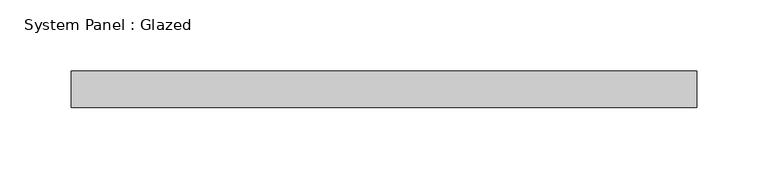
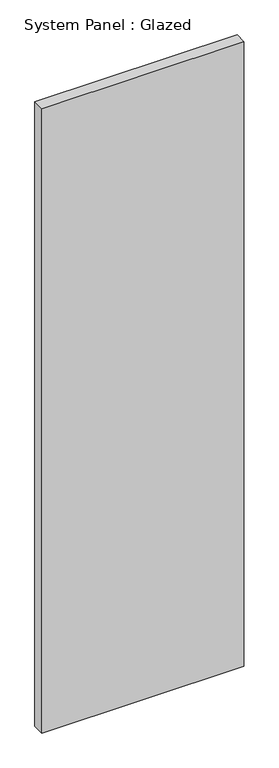
"""IFC4 building model written with IfcOpenShell, lengths in millimetres: plate geometry, System Panel : Glazed."""

from ifc_helpers import new_model, si_unit, origin, origin_with_axes, place, context, project, spatial, polyline, outline, extrude, source, transform, mapped, element, save


def system_panel_glazed_5472c3c5(model_context):
    return source(origin(), model_context, "Body", "SweptSolid", [
        extrude(outline(polyline([(219.075, 19.05), (-219.075, 19.05), (-219.075, 44.45), (219.075, 44.45), (219.075, 19.05)])), origin_with_axes(), (0.0, 0.0, 1.0), 1430.357611),
    ])


if __name__ == "__main__":
    model = new_model("IFC4")
    model_context = context("Model", 3, world=origin())
    ifc_project = project(units=[si_unit("LENGTHUNIT", "METRE", prefix="MILLI")], contexts=[model_context])
    site = spatial("IfcSite", under=ifc_project)
    building = spatial("IfcBuilding", under=site)
    placement = place(None, origin())
    system_panel_glazed_shape = system_panel_glazed_5472c3c5(model_context)
    element("IfcPlate", 1, ObjectType="System Panel : Glazed", at=placement, inside=building, context=model_context, shape_type="MappedRepresentation", body=[
        mapped(system_panel_glazed_shape, transform((0.0, 0.0, 0.0), x_axis=(1.0, 0.0, 0.0), y_axis=(0.0, 1.0, 0.0), z_axis=(0.0, 0.0, 1.0))),
    ])
    save(model, "model.ifc")

# Revit data of these elements
# Type "System Panel : Glazed"
#   Construction Type Id = "GSP4R"
#   Analytic Construction = "1/8 in Pilkington single glazing"
#   Visual Light Transmittance = 0.9
#   Solar Heat Gain Coefficient = 0.86
#   Heat Transfer Coefficient (U) = 1.18115 BTU/(h·ft²·°F)
#   Define Thermal Properties by = 1
# Element 1 (IfcPlate, "System Panel : Glazed")
#   Materials on its faces: "Glass"
# Materials
#   "Glass": class "Glass", colour RGB 0 128 192, transparency 0.75, Description = "Soda Lime Glass", Cost = 0
